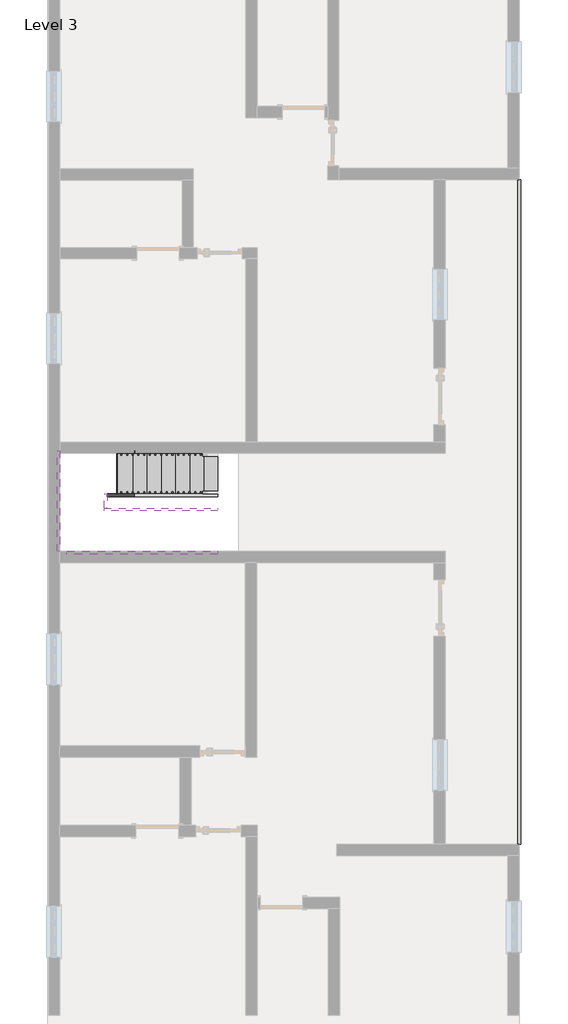
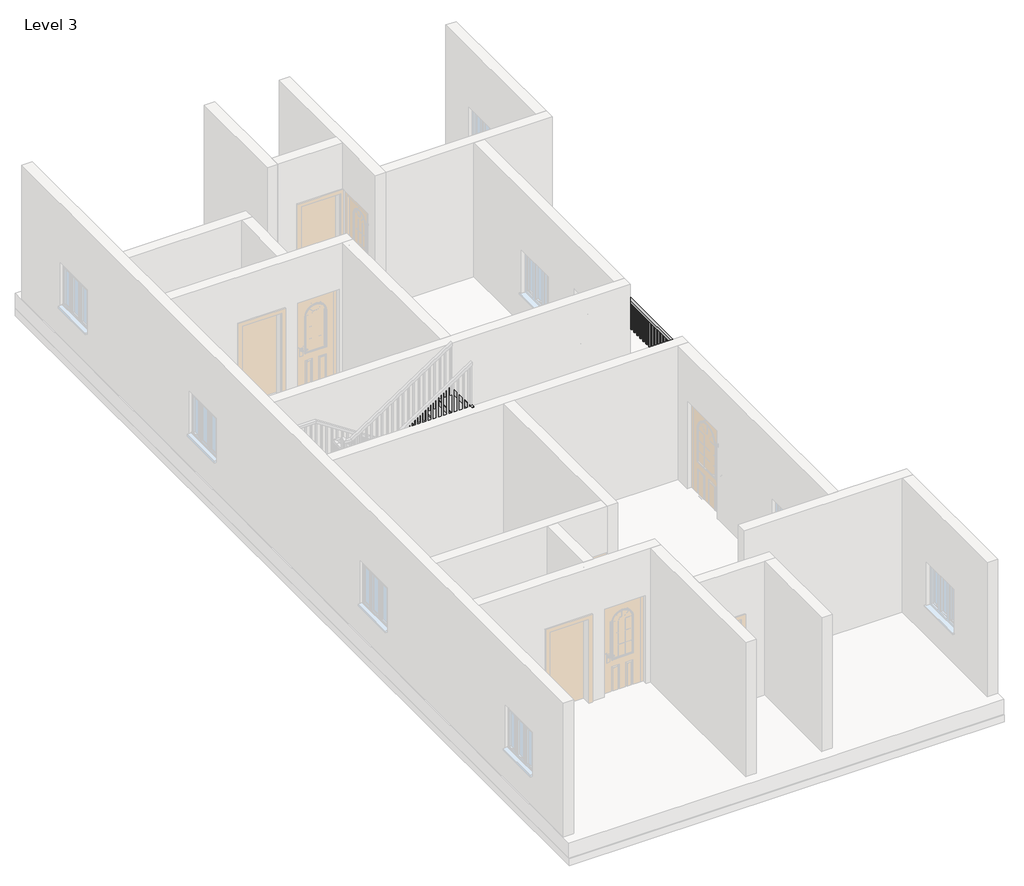
# One storey, part 3 of 3: 6 members, 1 railing, 1 stair flight.
"""IFC4 building model written with IfcOpenShell, lengths in millimetres."""

from ifc_helpers import new_model, si_unit, frame, origin, place, context, project, spatial, polyline, outline, extrude, transform, mapped, element, save
from components import stair_flight_e970c3af

model = new_model("IFC4")

# Units and contexts
model_context = context("Model", 3, world=origin())
ifc_project = project(units=[si_unit("LENGTHUNIT", "METRE", prefix="MILLI")], contexts=[model_context])

# Site, building, storey
site = spatial("IfcSite", under=ifc_project)
building = spatial("IfcBuilding", under=site)
storey = spatial("IfcBuildingStorey", under=building, Name="Level 3", Elevation=6096.0)

# Members
placement = place(None, origin())
element("IfcMember", 1, ObjectType="Stringer - 2\" Width", at=placement, inside=storey, context=model_context, shape_type="SweptSolid", body=[
    extrude(outline(polyline([(6096.0, -2118.1728655), (6313.4747739, -2118.1728655), (7623.2681072, -4099.3728655), (7257.8806735, -4099.3728655), (6096.0, -2341.9063005), (6096.0, -2118.1728655)])), frame((0.0, 417.8797121, 0.0), z_axis=(0.0, 1.0, 0.0), x_axis=(0.0, 0.0, 1.0)), (0.0, 0.0, 1.0), 50.8),
])
element("IfcMember", 2, ObjectType="Stringer - 2\" Width", at=placement, inside=storey, context=model_context, shape_type="SweptSolid", body=[
    extrude(outline(polyline([(-4150.1728655, 468.6797121), (-4099.3728655, 468.6797121), (-4099.3728655, 214.6797121), (-4150.1728655, 214.6797121), (-4150.1728655, 468.6797121)])), frame((0.0, 0.0, 7378.7), z_axis=(0.0, 0.0, 1.0), x_axis=(1.0, 0.0, 0.0)), (0.0, 0.0, 1.0), 304.8),
])
element("IfcMember", 3, ObjectType="Stringer - 2\" Width", at=placement, inside=storey, context=model_context, shape_type="SweptSolid", body=[
    extrude(outline(polyline([(7824.7747739, -4150.1728655), (7459.3873402, -4150.1728655), (8802.765118, -2118.1728655), (9168.1525517, -2118.1728655), (7824.7747739, -4150.1728655)])), frame((0.0, 163.8797121, 0.0), z_axis=(0.0, 1.0, 0.0), x_axis=(0.0, 0.0, 1.0)), (0.0, 0.0, 1.0), 50.8),
])
element("IfcMember", 4, ObjectType="Stringer - 2\" Width", at=placement, inside=storey, context=model_context, shape_type="SweptSolid", body=[
    extrude(outline(polyline([(6096.0, -2118.1728655), (6313.4747739, -2118.1728655), (7683.5, -4190.4799301), (7683.5, -4743.1668047), (6096.0, -2341.9063005), (6096.0, -2118.1728655)])), frame((0.0, 1192.5797121, 0.0), z_axis=(0.0, 1.0, 0.0), x_axis=(0.0, 0.0, 1.0)), (0.0, 0.0, 1.0), 50.8),
])
element("IfcMember", 5, ObjectType="Stringer - 2\" Width", at=placement, inside=storey, context=model_context, shape_type="SweptSolid", body=[
    extrude(outline(polyline([(-4994.7394105, 1243.3797121), (-4943.9394105, 1243.3797121), (-4943.9394105, -560.0202879), (-4994.7394105, -560.0202879), (-4994.7394105, 1243.3797121)])), frame((0.0, 0.0, 7378.7), z_axis=(0.0, 0.0, 1.0), x_axis=(1.0, 0.0, 0.0)), (0.0, 0.0, 1.0), 304.8),
])
element("IfcMember", 6, ObjectType="Stringer - 2\" Width", at=placement, inside=storey, context=model_context, shape_type="SweptSolid", body=[
    extrude(outline(polyline([(7378.7, -4272.2209431), (8802.765118, -2118.1728655), (9168.1525517, -2118.1728655), (7378.7, -4824.9078176), (7378.7, -4272.2209431)])), frame((0.0, -610.8202879, 0.0), z_axis=(0.0, 1.0, 0.0), x_axis=(0.0, 0.0, 1.0)), (0.0, 0.0, 1.0), 50.8),
])

# Railing
element("IfcRailing", 7, ObjectType="Handrail - Rectangular", at=placement, inside=storey, context=model_context, shape_type="SweptSolid", body=[
    extrude(outline(polyline([(3298.3605895, -5805.1202879), (3247.5605895, -5805.1202879), (3247.5605895, 6094.2483916), (3298.3605895, 6094.2483916), (3298.3605895, -5805.1202879)])), frame((0.0, 0.0, 6959.6), z_axis=(0.0, 0.0, 1.0), x_axis=(1.0, 0.0, 0.0)), (0.0, 0.0, 1.0), 50.8),
    extrude(outline(polyline([(3282.4855895, 6072.5547121), (3263.4355895, 6072.5547121), (3263.4355895, 6091.6047121), (3282.4855895, 6091.6047121), (3282.4855895, 6072.5547121)])), frame((0.0, 0.0, 6096.0), z_axis=(0.0, 0.0, 1.0), x_axis=(1.0, 0.0, 0.0)), (0.0, 0.0, 1.0), 863.6),
    extrude(outline(polyline([(3282.4855895, 5970.9547121), (3263.4355895, 5970.9547121), (3263.4355895, 5990.0047121), (3282.4855895, 5990.0047121), (3282.4855895, 5970.9547121)])), frame((0.0, 0.0, 6096.0), z_axis=(0.0, 0.0, 1.0), x_axis=(1.0, 0.0, 0.0)), (0.0, 0.0, 1.0), 863.6),
    extrude(outline(polyline([(3282.4855895, 5869.3547121), (3263.4355895, 5869.3547121), (3263.4355895, 5888.4047121), (3282.4855895, 5888.4047121), (3282.4855895, 5869.3547121)])), frame((0.0, 0.0, 6096.0), z_axis=(0.0, 0.0, 1.0), x_axis=(1.0, 0.0, 0.0)), (0.0, 0.0, 1.0), 863.6),
    extrude(outline(polyline([(3282.4855895, 5767.7547121), (3263.4355895, 5767.7547121), (3263.4355895, 5786.8047121), (3282.4855895, 5786.8047121), (3282.4855895, 5767.7547121)])), frame((0.0, 0.0, 6096.0), z_axis=(0.0, 0.0, 1.0), x_axis=(1.0, 0.0, 0.0)), (0.0, 0.0, 1.0), 863.6),
    extrude(outline(polyline([(3282.4855895, 5666.1547121), (3263.4355895, 5666.1547121), (3263.4355895, 5685.2047121), (3282.4855895, 5685.2047121), (3282.4855895, 5666.1547121)])), frame((0.0, 0.0, 6096.0), z_axis=(0.0, 0.0, 1.0), x_axis=(1.0, 0.0, 0.0)), (0.0, 0.0, 1.0), 863.6),
    extrude(outline(polyline([(3282.4855895, 5564.5547121), (3263.4355895, 5564.5547121), (3263.4355895, 5583.6047121), (3282.4855895, 5583.6047121), (3282.4855895, 5564.5547121)])), frame((0.0, 0.0, 6096.0), z_axis=(0.0, 0.0, 1.0), x_axis=(1.0, 0.0, 0.0)), (0.0, 0.0, 1.0), 863.6),
    extrude(outline(polyline([(3282.4855895, 5462.9547121), (3263.4355895, 5462.9547121), (3263.4355895, 5482.0047121), (3282.4855895, 5482.0047121), (3282.4855895, 5462.9547121)])), frame((0.0, 0.0, 6096.0), z_axis=(0.0, 0.0, 1.0), x_axis=(1.0, 0.0, 0.0)), (0.0, 0.0, 1.0), 863.6),
    extrude(outline(polyline([(3282.4855895, 5361.3547121), (3263.4355895, 5361.3547121), (3263.4355895, 5380.4047121), (3282.4855895, 5380.4047121), (3282.4855895, 5361.3547121)])), frame((0.0, 0.0, 6096.0), z_axis=(0.0, 0.0, 1.0), x_axis=(1.0, 0.0, 0.0)), (0.0, 0.0, 1.0), 863.6),
    extrude(outline(polyline([(3282.4855895, 5259.7547121), (3263.4355895, 5259.7547121), (3263.4355895, 5278.8047121), (3282.4855895, 5278.8047121), (3282.4855895, 5259.7547121)])), frame((0.0, 0.0, 6096.0), z_axis=(0.0, 0.0, 1.0), x_axis=(1.0, 0.0, 0.0)), (0.0, 0.0, 1.0), 863.6),
    extrude(outline(polyline([(3282.4855895, 5158.1547121), (3263.4355895, 5158.1547121), (3263.4355895, 5177.2047121), (3282.4855895, 5177.2047121), (3282.4855895, 5158.1547121)])), frame((0.0, 0.0, 6096.0), z_axis=(0.0, 0.0, 1.0), x_axis=(1.0, 0.0, 0.0)), (0.0, 0.0, 1.0), 863.6),
    extrude(outline(polyline([(3282.4855895, 5056.5547121), (3263.4355895, 5056.5547121), (3263.4355895, 5075.6047121), (3282.4855895, 5075.6047121), (3282.4855895, 5056.5547121)])), frame((0.0, 0.0, 6096.0), z_axis=(0.0, 0.0, 1.0), x_axis=(1.0, 0.0, 0.0)), (0.0, 0.0, 1.0), 863.6),
    extrude(outline(polyline([(3282.4855895, 4954.9547121), (3263.4355895, 4954.9547121), (3263.4355895, 4974.0047121), (3282.4855895, 4974.0047121), (3282.4855895, 4954.9547121)])), frame((0.0, 0.0, 6096.0), z_axis=(0.0, 0.0, 1.0), x_axis=(1.0, 0.0, 0.0)), (0.0, 0.0, 1.0), 863.6),
    extrude(outline(polyline([(3282.4855895, 4853.3547121), (3263.4355895, 4853.3547121), (3263.4355895, 4872.4047121), (3282.4855895, 4872.4047121), (3282.4855895, 4853.3547121)])), frame((0.0, 0.0, 6096.0), z_axis=(0.0, 0.0, 1.0), x_axis=(1.0, 0.0, 0.0)), (0.0, 0.0, 1.0), 863.6),
    extrude(outline(polyline([(3282.4855895, 4751.7547121), (3263.4355895, 4751.7547121), (3263.4355895, 4770.8047121), (3282.4855895, 4770.8047121), (3282.4855895, 4751.7547121)])), frame((0.0, 0.0, 6096.0), z_axis=(0.0, 0.0, 1.0), x_axis=(1.0, 0.0, 0.0)), (0.0, 0.0, 1.0), 863.6),
    extrude(outline(polyline([(3282.4855895, 4650.1547121), (3263.4355895, 4650.1547121), (3263.4355895, 4669.2047121), (3282.4855895, 4669.2047121), (3282.4855895, 4650.1547121)])), frame((0.0, 0.0, 6096.0), z_axis=(0.0, 0.0, 1.0), x_axis=(1.0, 0.0, 0.0)), (0.0, 0.0, 1.0), 863.6),
    extrude(outline(polyline([(3282.4855895, 4548.5547121), (3263.4355895, 4548.5547121), (3263.4355895, 4567.6047121), (3282.4855895, 4567.6047121), (3282.4855895, 4548.5547121)])), frame((0.0, 0.0, 6096.0), z_axis=(0.0, 0.0, 1.0), x_axis=(1.0, 0.0, 0.0)), (0.0, 0.0, 1.0), 863.6),
    extrude(outline(polyline([(3282.4855895, 4446.9547121), (3263.4355895, 4446.9547121), (3263.4355895, 4466.0047121), (3282.4855895, 4466.0047121), (3282.4855895, 4446.9547121)])), frame((0.0, 0.0, 6096.0), z_axis=(0.0, 0.0, 1.0), x_axis=(1.0, 0.0, 0.0)), (0.0, 0.0, 1.0), 863.6),
    extrude(outline(polyline([(3282.4855895, 4345.3547121), (3263.4355895, 4345.3547121), (3263.4355895, 4364.4047121), (3282.4855895, 4364.4047121), (3282.4855895, 4345.3547121)])), frame((0.0, 0.0, 6096.0), z_axis=(0.0, 0.0, 1.0), x_axis=(1.0, 0.0, 0.0)), (0.0, 0.0, 1.0), 863.6),
    extrude(outline(polyline([(3282.4855895, 4243.7547121), (3263.4355895, 4243.7547121), (3263.4355895, 4262.8047121), (3282.4855895, 4262.8047121), (3282.4855895, 4243.7547121)])), frame((0.0, 0.0, 6096.0), z_axis=(0.0, 0.0, 1.0), x_axis=(1.0, 0.0, 0.0)), (0.0, 0.0, 1.0), 863.6),
    extrude(outline(polyline([(3282.4855895, 4142.1547121), (3263.4355895, 4142.1547121), (3263.4355895, 4161.2047121), (3282.4855895, 4161.2047121), (3282.4855895, 4142.1547121)])), frame((0.0, 0.0, 6096.0), z_axis=(0.0, 0.0, 1.0), x_axis=(1.0, 0.0, 0.0)), (0.0, 0.0, 1.0), 863.6),
    extrude(outline(polyline([(3282.4855895, 4040.5547121), (3263.4355895, 4040.5547121), (3263.4355895, 4059.6047121), (3282.4855895, 4059.6047121), (3282.4855895, 4040.5547121)])), frame((0.0, 0.0, 6096.0), z_axis=(0.0, 0.0, 1.0), x_axis=(1.0, 0.0, 0.0)), (0.0, 0.0, 1.0), 863.6),
    extrude(outline(polyline([(3282.4855895, 3938.9547121), (3263.4355895, 3938.9547121), (3263.4355895, 3958.0047121), (3282.4855895, 3958.0047121), (3282.4855895, 3938.9547121)])), frame((0.0, 0.0, 6096.0), z_axis=(0.0, 0.0, 1.0), x_axis=(1.0, 0.0, 0.0)), (0.0, 0.0, 1.0), 863.6),
    extrude(outline(polyline([(3282.4855895, 3837.3547121), (3263.4355895, 3837.3547121), (3263.4355895, 3856.4047121), (3282.4855895, 3856.4047121), (3282.4855895, 3837.3547121)])), frame((0.0, 0.0, 6096.0), z_axis=(0.0, 0.0, 1.0), x_axis=(1.0, 0.0, 0.0)), (0.0, 0.0, 1.0), 863.6),
    extrude(outline(polyline([(3282.4855895, 3735.7547121), (3263.4355895, 3735.7547121), (3263.4355895, 3754.8047121), (3282.4855895, 3754.8047121), (3282.4855895, 3735.7547121)])), frame((0.0, 0.0, 6096.0), z_axis=(0.0, 0.0, 1.0), x_axis=(1.0, 0.0, 0.0)), (0.0, 0.0, 1.0), 863.6),
    extrude(outline(polyline([(3282.4855895, 3634.1547121), (3263.4355895, 3634.1547121), (3263.4355895, 3653.2047121), (3282.4855895, 3653.2047121), (3282.4855895, 3634.1547121)])), frame((0.0, 0.0, 6096.0), z_axis=(0.0, 0.0, 1.0), x_axis=(1.0, 0.0, 0.0)), (0.0, 0.0, 1.0), 863.6),
    extrude(outline(polyline([(3282.4855895, 3532.5547121), (3263.4355895, 3532.5547121), (3263.4355895, 3551.6047121), (3282.4855895, 3551.6047121), (3282.4855895, 3532.5547121)])), frame((0.0, 0.0, 6096.0), z_axis=(0.0, 0.0, 1.0), x_axis=(1.0, 0.0, 0.0)), (0.0, 0.0, 1.0), 863.6),
    extrude(outline(polyline([(3282.4855895, 3430.9547121), (3263.4355895, 3430.9547121), (3263.4355895, 3450.0047121), (3282.4855895, 3450.0047121), (3282.4855895, 3430.9547121)])), frame((0.0, 0.0, 6096.0), z_axis=(0.0, 0.0, 1.0), x_axis=(1.0, 0.0, 0.0)), (0.0, 0.0, 1.0), 863.6),
    extrude(outline(polyline([(3282.4855895, 3329.3547121), (3263.4355895, 3329.3547121), (3263.4355895, 3348.4047121), (3282.4855895, 3348.4047121), (3282.4855895, 3329.3547121)])), frame((0.0, 0.0, 6096.0), z_axis=(0.0, 0.0, 1.0), x_axis=(1.0, 0.0, 0.0)), (0.0, 0.0, 1.0), 863.6),
    extrude(outline(polyline([(3282.4855895, 3227.7547121), (3263.4355895, 3227.7547121), (3263.4355895, 3246.8047121), (3282.4855895, 3246.8047121), (3282.4855895, 3227.7547121)])), frame((0.0, 0.0, 6096.0), z_axis=(0.0, 0.0, 1.0), x_axis=(1.0, 0.0, 0.0)), (0.0, 0.0, 1.0), 863.6),
    extrude(outline(polyline([(3282.4855895, 3126.1547121), (3263.4355895, 3126.1547121), (3263.4355895, 3145.2047121), (3282.4855895, 3145.2047121), (3282.4855895, 3126.1547121)])), frame((0.0, 0.0, 6096.0), z_axis=(0.0, 0.0, 1.0), x_axis=(1.0, 0.0, 0.0)), (0.0, 0.0, 1.0), 863.6),
    extrude(outline(polyline([(3282.4855895, 3024.5547121), (3263.4355895, 3024.5547121), (3263.4355895, 3043.6047121), (3282.4855895, 3043.6047121), (3282.4855895, 3024.5547121)])), frame((0.0, 0.0, 6096.0), z_axis=(0.0, 0.0, 1.0), x_axis=(1.0, 0.0, 0.0)), (0.0, 0.0, 1.0), 863.6),
    extrude(outline(polyline([(3282.4855895, 2922.9547121), (3263.4355895, 2922.9547121), (3263.4355895, 2942.0047121), (3282.4855895, 2942.0047121), (3282.4855895, 2922.9547121)])), frame((0.0, 0.0, 6096.0), z_axis=(0.0, 0.0, 1.0), x_axis=(1.0, 0.0, 0.0)), (0.0, 0.0, 1.0), 863.6),
    extrude(outline(polyline([(3282.4855895, 2821.3547121), (3263.4355895, 2821.3547121), (3263.4355895, 2840.4047121), (3282.4855895, 2840.4047121), (3282.4855895, 2821.3547121)])), frame((0.0, 0.0, 6096.0), z_axis=(0.0, 0.0, 1.0), x_axis=(1.0, 0.0, 0.0)), (0.0, 0.0, 1.0), 863.6),
    extrude(outline(polyline([(3282.4855895, 2719.7547121), (3263.4355895, 2719.7547121), (3263.4355895, 2738.8047121), (3282.4855895, 2738.8047121), (3282.4855895, 2719.7547121)])), frame((0.0, 0.0, 6096.0), z_axis=(0.0, 0.0, 1.0), x_axis=(1.0, 0.0, 0.0)), (0.0, 0.0, 1.0), 863.6),
    extrude(outline(polyline([(3282.4855895, 2618.1547121), (3263.4355895, 2618.1547121), (3263.4355895, 2637.2047121), (3282.4855895, 2637.2047121), (3282.4855895, 2618.1547121)])), frame((0.0, 0.0, 6096.0), z_axis=(0.0, 0.0, 1.0), x_axis=(1.0, 0.0, 0.0)), (0.0, 0.0, 1.0), 863.6),
    extrude(outline(polyline([(3282.4855895, 2516.5547121), (3263.4355895, 2516.5547121), (3263.4355895, 2535.6047121), (3282.4855895, 2535.6047121), (3282.4855895, 2516.5547121)])), frame((0.0, 0.0, 6096.0), z_axis=(0.0, 0.0, 1.0), x_axis=(1.0, 0.0, 0.0)), (0.0, 0.0, 1.0), 863.6),
    extrude(outline(polyline([(3282.4855895, 2414.9547121), (3263.4355895, 2414.9547121), (3263.4355895, 2434.0047121), (3282.4855895, 2434.0047121), (3282.4855895, 2414.9547121)])), frame((0.0, 0.0, 6096.0), z_axis=(0.0, 0.0, 1.0), x_axis=(1.0, 0.0, 0.0)), (0.0, 0.0, 1.0), 863.6),
    extrude(outline(polyline([(3282.4855895, 2313.3547121), (3263.4355895, 2313.3547121), (3263.4355895, 2332.4047121), (3282.4855895, 2332.4047121), (3282.4855895, 2313.3547121)])), frame((0.0, 0.0, 6096.0), z_axis=(0.0, 0.0, 1.0), x_axis=(1.0, 0.0, 0.0)), (0.0, 0.0, 1.0), 863.6),
    extrude(outline(polyline([(3282.4855895, 2211.7547121), (3263.4355895, 2211.7547121), (3263.4355895, 2230.8047121), (3282.4855895, 2230.8047121), (3282.4855895, 2211.7547121)])), frame((0.0, 0.0, 6096.0), z_axis=(0.0, 0.0, 1.0), x_axis=(1.0, 0.0, 0.0)), (0.0, 0.0, 1.0), 863.6),
    extrude(outline(polyline([(3282.4855895, 2110.1547121), (3263.4355895, 2110.1547121), (3263.4355895, 2129.2047121), (3282.4855895, 2129.2047121), (3282.4855895, 2110.1547121)])), frame((0.0, 0.0, 6096.0), z_axis=(0.0, 0.0, 1.0), x_axis=(1.0, 0.0, 0.0)), (0.0, 0.0, 1.0), 863.6),
    extrude(outline(polyline([(3282.4855895, 2008.5547121), (3263.4355895, 2008.5547121), (3263.4355895, 2027.6047121), (3282.4855895, 2027.6047121), (3282.4855895, 2008.5547121)])), frame((0.0, 0.0, 6096.0), z_axis=(0.0, 0.0, 1.0), x_axis=(1.0, 0.0, 0.0)), (0.0, 0.0, 1.0), 863.6),
    extrude(outline(polyline([(3282.4855895, 1906.9547121), (3263.4355895, 1906.9547121), (3263.4355895, 1926.0047121), (3282.4855895, 1926.0047121), (3282.4855895, 1906.9547121)])), frame((0.0, 0.0, 6096.0), z_axis=(0.0, 0.0, 1.0), x_axis=(1.0, 0.0, 0.0)), (0.0, 0.0, 1.0), 863.6),
    extrude(outline(polyline([(3282.4855895, 1805.3547121), (3263.4355895, 1805.3547121), (3263.4355895, 1824.4047121), (3282.4855895, 1824.4047121), (3282.4855895, 1805.3547121)])), frame((0.0, 0.0, 6096.0), z_axis=(0.0, 0.0, 1.0), x_axis=(1.0, 0.0, 0.0)), (0.0, 0.0, 1.0), 863.6),
    extrude(outline(polyline([(3282.4855895, 1703.7547121), (3263.4355895, 1703.7547121), (3263.4355895, 1722.8047121), (3282.4855895, 1722.8047121), (3282.4855895, 1703.7547121)])), frame((0.0, 0.0, 6096.0), z_axis=(0.0, 0.0, 1.0), x_axis=(1.0, 0.0, 0.0)), (0.0, 0.0, 1.0), 863.6),
    extrude(outline(polyline([(3282.4855895, 1602.1547121), (3263.4355895, 1602.1547121), (3263.4355895, 1621.2047121), (3282.4855895, 1621.2047121), (3282.4855895, 1602.1547121)])), frame((0.0, 0.0, 6096.0), z_axis=(0.0, 0.0, 1.0), x_axis=(1.0, 0.0, 0.0)), (0.0, 0.0, 1.0), 863.6),
    extrude(outline(polyline([(3282.4855895, 1500.5547121), (3263.4355895, 1500.5547121), (3263.4355895, 1519.6047121), (3282.4855895, 1519.6047121), (3282.4855895, 1500.5547121)])), frame((0.0, 0.0, 6096.0), z_axis=(0.0, 0.0, 1.0), x_axis=(1.0, 0.0, 0.0)), (0.0, 0.0, 1.0), 863.6),
    extrude(outline(polyline([(3282.4855895, 1398.9547121), (3263.4355895, 1398.9547121), (3263.4355895, 1418.0047121), (3282.4855895, 1418.0047121), (3282.4855895, 1398.9547121)])), frame((0.0, 0.0, 6096.0), z_axis=(0.0, 0.0, 1.0), x_axis=(1.0, 0.0, 0.0)), (0.0, 0.0, 1.0), 863.6),
    extrude(outline(polyline([(3282.4855895, 1297.3547121), (3263.4355895, 1297.3547121), (3263.4355895, 1316.4047121), (3282.4855895, 1316.4047121), (3282.4855895, 1297.3547121)])), frame((0.0, 0.0, 6096.0), z_axis=(0.0, 0.0, 1.0), x_axis=(1.0, 0.0, 0.0)), (0.0, 0.0, 1.0), 863.6),
    extrude(outline(polyline([(3282.4855895, 1195.7547121), (3263.4355895, 1195.7547121), (3263.4355895, 1214.8047121), (3282.4855895, 1214.8047121), (3282.4855895, 1195.7547121)])), frame((0.0, 0.0, 6096.0), z_axis=(0.0, 0.0, 1.0), x_axis=(1.0, 0.0, 0.0)), (0.0, 0.0, 1.0), 863.6),
    extrude(outline(polyline([(3282.4855895, 1094.1547121), (3263.4355895, 1094.1547121), (3263.4355895, 1113.2047121), (3282.4855895, 1113.2047121), (3282.4855895, 1094.1547121)])), frame((0.0, 0.0, 6096.0), z_axis=(0.0, 0.0, 1.0), x_axis=(1.0, 0.0, 0.0)), (0.0, 0.0, 1.0), 863.6),
    extrude(outline(polyline([(3282.4855895, 992.5547121), (3263.4355895, 992.5547121), (3263.4355895, 1011.6047121), (3282.4855895, 1011.6047121), (3282.4855895, 992.5547121)])), frame((0.0, 0.0, 6096.0), z_axis=(0.0, 0.0, 1.0), x_axis=(1.0, 0.0, 0.0)), (0.0, 0.0, 1.0), 863.6),
    extrude(outline(polyline([(3282.4855895, 890.9547121), (3263.4355895, 890.9547121), (3263.4355895, 910.0047121), (3282.4855895, 910.0047121), (3282.4855895, 890.9547121)])), frame((0.0, 0.0, 6096.0), z_axis=(0.0, 0.0, 1.0), x_axis=(1.0, 0.0, 0.0)), (0.0, 0.0, 1.0), 863.6),
    extrude(outline(polyline([(3282.4855895, 789.3547121), (3263.4355895, 789.3547121), (3263.4355895, 808.4047121), (3282.4855895, 808.4047121), (3282.4855895, 789.3547121)])), frame((0.0, 0.0, 6096.0), z_axis=(0.0, 0.0, 1.0), x_axis=(1.0, 0.0, 0.0)), (0.0, 0.0, 1.0), 863.6),
    extrude(outline(polyline([(3282.4855895, 687.7547121), (3263.4355895, 687.7547121), (3263.4355895, 706.8047121), (3282.4855895, 706.8047121), (3282.4855895, 687.7547121)])), frame((0.0, 0.0, 6096.0), z_axis=(0.0, 0.0, 1.0), x_axis=(1.0, 0.0, 0.0)), (0.0, 0.0, 1.0), 863.6),
    extrude(outline(polyline([(3282.4855895, 586.1547121), (3263.4355895, 586.1547121), (3263.4355895, 605.2047121), (3282.4855895, 605.2047121), (3282.4855895, 586.1547121)])), frame((0.0, 0.0, 6096.0), z_axis=(0.0, 0.0, 1.0), x_axis=(1.0, 0.0, 0.0)), (0.0, 0.0, 1.0), 863.6),
    extrude(outline(polyline([(3282.4855895, 484.5547121), (3263.4355895, 484.5547121), (3263.4355895, 503.6047121), (3282.4855895, 503.6047121), (3282.4855895, 484.5547121)])), frame((0.0, 0.0, 6096.0), z_axis=(0.0, 0.0, 1.0), x_axis=(1.0, 0.0, 0.0)), (0.0, 0.0, 1.0), 863.6),
    extrude(outline(polyline([(3282.4855895, 382.9547121), (3263.4355895, 382.9547121), (3263.4355895, 402.0047121), (3282.4855895, 402.0047121), (3282.4855895, 382.9547121)])), frame((0.0, 0.0, 6096.0), z_axis=(0.0, 0.0, 1.0), x_axis=(1.0, 0.0, 0.0)), (0.0, 0.0, 1.0), 863.6),
    extrude(outline(polyline([(3282.4855895, 281.3547121), (3263.4355895, 281.3547121), (3263.4355895, 300.4047121), (3282.4855895, 300.4047121), (3282.4855895, 281.3547121)])), frame((0.0, 0.0, 6096.0), z_axis=(0.0, 0.0, 1.0), x_axis=(1.0, 0.0, 0.0)), (0.0, 0.0, 1.0), 863.6),
    extrude(outline(polyline([(3282.4855895, 179.7547121), (3263.4355895, 179.7547121), (3263.4355895, 198.8047121), (3282.4855895, 198.8047121), (3282.4855895, 179.7547121)])), frame((0.0, 0.0, 6096.0), z_axis=(0.0, 0.0, 1.0), x_axis=(1.0, 0.0, 0.0)), (0.0, 0.0, 1.0), 863.6),
    extrude(outline(polyline([(3282.4855895, 78.1547121), (3263.4355895, 78.1547121), (3263.4355895, 97.2047121), (3282.4855895, 97.2047121), (3282.4855895, 78.1547121)])), frame((0.0, 0.0, 6096.0), z_axis=(0.0, 0.0, 1.0), x_axis=(1.0, 0.0, 0.0)), (0.0, 0.0, 1.0), 863.6),
    extrude(outline(polyline([(3282.4855895, -23.4452879), (3263.4355895, -23.4452879), (3263.4355895, -4.3952879), (3282.4855895, -4.3952879), (3282.4855895, -23.4452879)])), frame((0.0, 0.0, 6096.0), z_axis=(0.0, 0.0, 1.0), x_axis=(1.0, 0.0, 0.0)), (0.0, 0.0, 1.0), 863.6),
    extrude(outline(polyline([(3282.4855895, -125.0452879), (3263.4355895, -125.0452879), (3263.4355895, -105.9952879), (3282.4855895, -105.9952879), (3282.4855895, -125.0452879)])), frame((0.0, 0.0, 6096.0), z_axis=(0.0, 0.0, 1.0), x_axis=(1.0, 0.0, 0.0)), (0.0, 0.0, 1.0), 863.6),
    extrude(outline(polyline([(3282.4855895, -226.6452879), (3263.4355895, -226.6452879), (3263.4355895, -207.5952879), (3282.4855895, -207.5952879), (3282.4855895, -226.6452879)])), frame((0.0, 0.0, 6096.0), z_axis=(0.0, 0.0, 1.0), x_axis=(1.0, 0.0, 0.0)), (0.0, 0.0, 1.0), 863.6),
    extrude(outline(polyline([(3282.4855895, -328.2452879), (3263.4355895, -328.2452879), (3263.4355895, -309.1952879), (3282.4855895, -309.1952879), (3282.4855895, -328.2452879)])), frame((0.0, 0.0, 6096.0), z_axis=(0.0, 0.0, 1.0), x_axis=(1.0, 0.0, 0.0)), (0.0, 0.0, 1.0), 863.6),
    extrude(outline(polyline([(3282.4855895, -429.8452879), (3263.4355895, -429.8452879), (3263.4355895, -410.7952879), (3282.4855895, -410.7952879), (3282.4855895, -429.8452879)])), frame((0.0, 0.0, 6096.0), z_axis=(0.0, 0.0, 1.0), x_axis=(1.0, 0.0, 0.0)), (0.0, 0.0, 1.0), 863.6),
    extrude(outline(polyline([(3282.4855895, -531.4452879), (3263.4355895, -531.4452879), (3263.4355895, -512.3952879), (3282.4855895, -512.3952879), (3282.4855895, -531.4452879)])), frame((0.0, 0.0, 6096.0), z_axis=(0.0, 0.0, 1.0), x_axis=(1.0, 0.0, 0.0)), (0.0, 0.0, 1.0), 863.6),
    extrude(outline(polyline([(3282.4855895, -633.0452879), (3263.4355895, -633.0452879), (3263.4355895, -613.9952879), (3282.4855895, -613.9952879), (3282.4855895, -633.0452879)])), frame((0.0, 0.0, 6096.0), z_axis=(0.0, 0.0, 1.0), x_axis=(1.0, 0.0, 0.0)), (0.0, 0.0, 1.0), 863.6),
    extrude(outline(polyline([(3282.4855895, -734.6452879), (3263.4355895, -734.6452879), (3263.4355895, -715.5952879), (3282.4855895, -715.5952879), (3282.4855895, -734.6452879)])), frame((0.0, 0.0, 6096.0), z_axis=(0.0, 0.0, 1.0), x_axis=(1.0, 0.0, 0.0)), (0.0, 0.0, 1.0), 863.6),
    extrude(outline(polyline([(3282.4855895, -836.2452879), (3263.4355895, -836.2452879), (3263.4355895, -817.1952879), (3282.4855895, -817.1952879), (3282.4855895, -836.2452879)])), frame((0.0, 0.0, 6096.0), z_axis=(0.0, 0.0, 1.0), x_axis=(1.0, 0.0, 0.0)), (0.0, 0.0, 1.0), 863.6),
    extrude(outline(polyline([(3282.4855895, -937.8452879), (3263.4355895, -937.8452879), (3263.4355895, -918.7952879), (3282.4855895, -918.7952879), (3282.4855895, -937.8452879)])), frame((0.0, 0.0, 6096.0), z_axis=(0.0, 0.0, 1.0), x_axis=(1.0, 0.0, 0.0)), (0.0, 0.0, 1.0), 863.6),
    extrude(outline(polyline([(3282.4855895, -1039.4452879), (3263.4355895, -1039.4452879), (3263.4355895, -1020.3952879), (3282.4855895, -1020.3952879), (3282.4855895, -1039.4452879)])), frame((0.0, 0.0, 6096.0), z_axis=(0.0, 0.0, 1.0), x_axis=(1.0, 0.0, 0.0)), (0.0, 0.0, 1.0), 863.6),
    extrude(outline(polyline([(3282.4855895, -1141.0452879), (3263.4355895, -1141.0452879), (3263.4355895, -1121.9952879), (3282.4855895, -1121.9952879), (3282.4855895, -1141.0452879)])), frame((0.0, 0.0, 6096.0), z_axis=(0.0, 0.0, 1.0), x_axis=(1.0, 0.0, 0.0)), (0.0, 0.0, 1.0), 863.6),
    extrude(outline(polyline([(3282.4855895, -1242.6452879), (3263.4355895, -1242.6452879), (3263.4355895, -1223.5952879), (3282.4855895, -1223.5952879), (3282.4855895, -1242.6452879)])), frame((0.0, 0.0, 6096.0), z_axis=(0.0, 0.0, 1.0), x_axis=(1.0, 0.0, 0.0)), (0.0, 0.0, 1.0), 863.6),
    extrude(outline(polyline([(3282.4855895, -1344.2452879), (3263.4355895, -1344.2452879), (3263.4355895, -1325.1952879), (3282.4855895, -1325.1952879), (3282.4855895, -1344.2452879)])), frame((0.0, 0.0, 6096.0), z_axis=(0.0, 0.0, 1.0), x_axis=(1.0, 0.0, 0.0)), (0.0, 0.0, 1.0), 863.6),
    extrude(outline(polyline([(3282.4855895, -1445.8452879), (3263.4355895, -1445.8452879), (3263.4355895, -1426.7952879), (3282.4855895, -1426.7952879), (3282.4855895, -1445.8452879)])), frame((0.0, 0.0, 6096.0), z_axis=(0.0, 0.0, 1.0), x_axis=(1.0, 0.0, 0.0)), (0.0, 0.0, 1.0), 863.6),
    extrude(outline(polyline([(3282.4855895, -1547.4452879), (3263.4355895, -1547.4452879), (3263.4355895, -1528.3952879), (3282.4855895, -1528.3952879), (3282.4855895, -1547.4452879)])), frame((0.0, 0.0, 6096.0), z_axis=(0.0, 0.0, 1.0), x_axis=(1.0, 0.0, 0.0)), (0.0, 0.0, 1.0), 863.6),
    extrude(outline(polyline([(3282.4855895, -1649.0452879), (3263.4355895, -1649.0452879), (3263.4355895, -1629.9952879), (3282.4855895, -1629.9952879), (3282.4855895, -1649.0452879)])), frame((0.0, 0.0, 6096.0), z_axis=(0.0, 0.0, 1.0), x_axis=(1.0, 0.0, 0.0)), (0.0, 0.0, 1.0), 863.6),
    extrude(outline(polyline([(3282.4855895, -1750.6452879), (3263.4355895, -1750.6452879), (3263.4355895, -1731.5952879), (3282.4855895, -1731.5952879), (3282.4855895, -1750.6452879)])), frame((0.0, 0.0, 6096.0), z_axis=(0.0, 0.0, 1.0), x_axis=(1.0, 0.0, 0.0)), (0.0, 0.0, 1.0), 863.6),
    extrude(outline(polyline([(3282.4855895, -1852.2452879), (3263.4355895, -1852.2452879), (3263.4355895, -1833.1952879), (3282.4855895, -1833.1952879), (3282.4855895, -1852.2452879)])), frame((0.0, 0.0, 6096.0), z_axis=(0.0, 0.0, 1.0), x_axis=(1.0, 0.0, 0.0)), (0.0, 0.0, 1.0), 863.6),
    extrude(outline(polyline([(3282.4855895, -1953.8452879), (3263.4355895, -1953.8452879), (3263.4355895, -1934.7952879), (3282.4855895, -1934.7952879), (3282.4855895, -1953.8452879)])), frame((0.0, 0.0, 6096.0), z_axis=(0.0, 0.0, 1.0), x_axis=(1.0, 0.0, 0.0)), (0.0, 0.0, 1.0), 863.6),
    extrude(outline(polyline([(3282.4855895, -2055.4452879), (3263.4355895, -2055.4452879), (3263.4355895, -2036.3952879), (3282.4855895, -2036.3952879), (3282.4855895, -2055.4452879)])), frame((0.0, 0.0, 6096.0), z_axis=(0.0, 0.0, 1.0), x_axis=(1.0, 0.0, 0.0)), (0.0, 0.0, 1.0), 863.6),
    extrude(outline(polyline([(3282.4855895, -2157.0452879), (3263.4355895, -2157.0452879), (3263.4355895, -2137.9952879), (3282.4855895, -2137.9952879), (3282.4855895, -2157.0452879)])), frame((0.0, 0.0, 6096.0), z_axis=(0.0, 0.0, 1.0), x_axis=(1.0, 0.0, 0.0)), (0.0, 0.0, 1.0), 863.6),
    extrude(outline(polyline([(3282.4855895, -2258.6452879), (3263.4355895, -2258.6452879), (3263.4355895, -2239.5952879), (3282.4855895, -2239.5952879), (3282.4855895, -2258.6452879)])), frame((0.0, 0.0, 6096.0), z_axis=(0.0, 0.0, 1.0), x_axis=(1.0, 0.0, 0.0)), (0.0, 0.0, 1.0), 863.6),
    extrude(outline(polyline([(3282.4855895, -2360.2452879), (3263.4355895, -2360.2452879), (3263.4355895, -2341.1952879), (3282.4855895, -2341.1952879), (3282.4855895, -2360.2452879)])), frame((0.0, 0.0, 6096.0), z_axis=(0.0, 0.0, 1.0), x_axis=(1.0, 0.0, 0.0)), (0.0, 0.0, 1.0), 863.6),
    extrude(outline(polyline([(3282.4855895, -2461.8452879), (3263.4355895, -2461.8452879), (3263.4355895, -2442.7952879), (3282.4855895, -2442.7952879), (3282.4855895, -2461.8452879)])), frame((0.0, 0.0, 6096.0), z_axis=(0.0, 0.0, 1.0), x_axis=(1.0, 0.0, 0.0)), (0.0, 0.0, 1.0), 863.6),
    extrude(outline(polyline([(3282.4855895, -2563.4452879), (3263.4355895, -2563.4452879), (3263.4355895, -2544.3952879), (3282.4855895, -2544.3952879), (3282.4855895, -2563.4452879)])), frame((0.0, 0.0, 6096.0), z_axis=(0.0, 0.0, 1.0), x_axis=(1.0, 0.0, 0.0)), (0.0, 0.0, 1.0), 863.6),
    extrude(outline(polyline([(3282.4855895, -2665.0452879), (3263.4355895, -2665.0452879), (3263.4355895, -2645.9952879), (3282.4855895, -2645.9952879), (3282.4855895, -2665.0452879)])), frame((0.0, 0.0, 6096.0), z_axis=(0.0, 0.0, 1.0), x_axis=(1.0, 0.0, 0.0)), (0.0, 0.0, 1.0), 863.6),
    extrude(outline(polyline([(3282.4855895, -2766.6452879), (3263.4355895, -2766.6452879), (3263.4355895, -2747.5952879), (3282.4855895, -2747.5952879), (3282.4855895, -2766.6452879)])), frame((0.0, 0.0, 6096.0), z_axis=(0.0, 0.0, 1.0), x_axis=(1.0, 0.0, 0.0)), (0.0, 0.0, 1.0), 863.6),
    extrude(outline(polyline([(3282.4855895, -2868.2452879), (3263.4355895, -2868.2452879), (3263.4355895, -2849.1952879), (3282.4855895, -2849.1952879), (3282.4855895, -2868.2452879)])), frame((0.0, 0.0, 6096.0), z_axis=(0.0, 0.0, 1.0), x_axis=(1.0, 0.0, 0.0)), (0.0, 0.0, 1.0), 863.6),
    extrude(outline(polyline([(3282.4855895, -2969.8452879), (3263.4355895, -2969.8452879), (3263.4355895, -2950.7952879), (3282.4855895, -2950.7952879), (3282.4855895, -2969.8452879)])), frame((0.0, 0.0, 6096.0), z_axis=(0.0, 0.0, 1.0), x_axis=(1.0, 0.0, 0.0)), (0.0, 0.0, 1.0), 863.6),
    extrude(outline(polyline([(3282.4855895, -3071.4452879), (3263.4355895, -3071.4452879), (3263.4355895, -3052.3952879), (3282.4855895, -3052.3952879), (3282.4855895, -3071.4452879)])), frame((0.0, 0.0, 6096.0), z_axis=(0.0, 0.0, 1.0), x_axis=(1.0, 0.0, 0.0)), (0.0, 0.0, 1.0), 863.6),
    extrude(outline(polyline([(3282.4855895, -3173.0452879), (3263.4355895, -3173.0452879), (3263.4355895, -3153.9952879), (3282.4855895, -3153.9952879), (3282.4855895, -3173.0452879)])), frame((0.0, 0.0, 6096.0), z_axis=(0.0, 0.0, 1.0), x_axis=(1.0, 0.0, 0.0)), (0.0, 0.0, 1.0), 863.6),
    extrude(outline(polyline([(3282.4855895, -3274.6452879), (3263.4355895, -3274.6452879), (3263.4355895, -3255.5952879), (3282.4855895, -3255.5952879), (3282.4855895, -3274.6452879)])), frame((0.0, 0.0, 6096.0), z_axis=(0.0, 0.0, 1.0), x_axis=(1.0, 0.0, 0.0)), (0.0, 0.0, 1.0), 863.6),
    extrude(outline(polyline([(3282.4855895, -3376.2452879), (3263.4355895, -3376.2452879), (3263.4355895, -3357.1952879), (3282.4855895, -3357.1952879), (3282.4855895, -3376.2452879)])), frame((0.0, 0.0, 6096.0), z_axis=(0.0, 0.0, 1.0), x_axis=(1.0, 0.0, 0.0)), (0.0, 0.0, 1.0), 863.6),
    extrude(outline(polyline([(3282.4855895, -3477.8452879), (3263.4355895, -3477.8452879), (3263.4355895, -3458.7952879), (3282.4855895, -3458.7952879), (3282.4855895, -3477.8452879)])), frame((0.0, 0.0, 6096.0), z_axis=(0.0, 0.0, 1.0), x_axis=(1.0, 0.0, 0.0)), (0.0, 0.0, 1.0), 863.6),
    extrude(outline(polyline([(3282.4855895, -3579.4452879), (3263.4355895, -3579.4452879), (3263.4355895, -3560.3952879), (3282.4855895, -3560.3952879), (3282.4855895, -3579.4452879)])), frame((0.0, 0.0, 6096.0), z_axis=(0.0, 0.0, 1.0), x_axis=(1.0, 0.0, 0.0)), (0.0, 0.0, 1.0), 863.6),
    extrude(outline(polyline([(3282.4855895, -3681.0452879), (3263.4355895, -3681.0452879), (3263.4355895, -3661.9952879), (3282.4855895, -3661.9952879), (3282.4855895, -3681.0452879)])), frame((0.0, 0.0, 6096.0), z_axis=(0.0, 0.0, 1.0), x_axis=(1.0, 0.0, 0.0)), (0.0, 0.0, 1.0), 863.6),
    extrude(outline(polyline([(3282.4855895, -3782.6452879), (3263.4355895, -3782.6452879), (3263.4355895, -3763.5952879), (3282.4855895, -3763.5952879), (3282.4855895, -3782.6452879)])), frame((0.0, 0.0, 6096.0), z_axis=(0.0, 0.0, 1.0), x_axis=(1.0, 0.0, 0.0)), (0.0, 0.0, 1.0), 863.6),
    extrude(outline(polyline([(3282.4855895, -3884.2452879), (3263.4355895, -3884.2452879), (3263.4355895, -3865.1952879), (3282.4855895, -3865.1952879), (3282.4855895, -3884.2452879)])), frame((0.0, 0.0, 6096.0), z_axis=(0.0, 0.0, 1.0), x_axis=(1.0, 0.0, 0.0)), (0.0, 0.0, 1.0), 863.6),
    extrude(outline(polyline([(3282.4855895, -3985.8452879), (3263.4355895, -3985.8452879), (3263.4355895, -3966.7952879), (3282.4855895, -3966.7952879), (3282.4855895, -3985.8452879)])), frame((0.0, 0.0, 6096.0), z_axis=(0.0, 0.0, 1.0), x_axis=(1.0, 0.0, 0.0)), (0.0, 0.0, 1.0), 863.6),
    extrude(outline(polyline([(3282.4855895, -4087.4452879), (3263.4355895, -4087.4452879), (3263.4355895, -4068.3952879), (3282.4855895, -4068.3952879), (3282.4855895, -4087.4452879)])), frame((0.0, 0.0, 6096.0), z_axis=(0.0, 0.0, 1.0), x_axis=(1.0, 0.0, 0.0)), (0.0, 0.0, 1.0), 863.6),
    extrude(outline(polyline([(3282.4855895, -4189.0452879), (3263.4355895, -4189.0452879), (3263.4355895, -4169.9952879), (3282.4855895, -4169.9952879), (3282.4855895, -4189.0452879)])), frame((0.0, 0.0, 6096.0), z_axis=(0.0, 0.0, 1.0), x_axis=(1.0, 0.0, 0.0)), (0.0, 0.0, 1.0), 863.6),
    extrude(outline(polyline([(3282.4855895, -4290.6452879), (3263.4355895, -4290.6452879), (3263.4355895, -4271.5952879), (3282.4855895, -4271.5952879), (3282.4855895, -4290.6452879)])), frame((0.0, 0.0, 6096.0), z_axis=(0.0, 0.0, 1.0), x_axis=(1.0, 0.0, 0.0)), (0.0, 0.0, 1.0), 863.6),
    extrude(outline(polyline([(3282.4855895, -4392.2452879), (3263.4355895, -4392.2452879), (3263.4355895, -4373.1952879), (3282.4855895, -4373.1952879), (3282.4855895, -4392.2452879)])), frame((0.0, 0.0, 6096.0), z_axis=(0.0, 0.0, 1.0), x_axis=(1.0, 0.0, 0.0)), (0.0, 0.0, 1.0), 863.6),
    extrude(outline(polyline([(3282.4855895, -4493.8452879), (3263.4355895, -4493.8452879), (3263.4355895, -4474.7952879), (3282.4855895, -4474.7952879), (3282.4855895, -4493.8452879)])), frame((0.0, 0.0, 6096.0), z_axis=(0.0, 0.0, 1.0), x_axis=(1.0, 0.0, 0.0)), (0.0, 0.0, 1.0), 863.6),
    extrude(outline(polyline([(3282.4855895, -4595.4452879), (3263.4355895, -4595.4452879), (3263.4355895, -4576.3952879), (3282.4855895, -4576.3952879), (3282.4855895, -4595.4452879)])), frame((0.0, 0.0, 6096.0), z_axis=(0.0, 0.0, 1.0), x_axis=(1.0, 0.0, 0.0)), (0.0, 0.0, 1.0), 863.6),
    extrude(outline(polyline([(3282.4855895, -4697.0452879), (3263.4355895, -4697.0452879), (3263.4355895, -4677.9952879), (3282.4855895, -4677.9952879), (3282.4855895, -4697.0452879)])), frame((0.0, 0.0, 6096.0), z_axis=(0.0, 0.0, 1.0), x_axis=(1.0, 0.0, 0.0)), (0.0, 0.0, 1.0), 863.6),
    extrude(outline(polyline([(3282.4855895, -4798.6452879), (3263.4355895, -4798.6452879), (3263.4355895, -4779.5952879), (3282.4855895, -4779.5952879), (3282.4855895, -4798.6452879)])), frame((0.0, 0.0, 6096.0), z_axis=(0.0, 0.0, 1.0), x_axis=(1.0, 0.0, 0.0)), (0.0, 0.0, 1.0), 863.6),
    extrude(outline(polyline([(3282.4855895, -4900.2452879), (3263.4355895, -4900.2452879), (3263.4355895, -4881.1952879), (3282.4855895, -4881.1952879), (3282.4855895, -4900.2452879)])), frame((0.0, 0.0, 6096.0), z_axis=(0.0, 0.0, 1.0), x_axis=(1.0, 0.0, 0.0)), (0.0, 0.0, 1.0), 863.6),
    extrude(outline(polyline([(3282.4855895, -5001.8452879), (3263.4355895, -5001.8452879), (3263.4355895, -4982.7952879), (3282.4855895, -4982.7952879), (3282.4855895, -5001.8452879)])), frame((0.0, 0.0, 6096.0), z_axis=(0.0, 0.0, 1.0), x_axis=(1.0, 0.0, 0.0)), (0.0, 0.0, 1.0), 863.6),
    extrude(outline(polyline([(3282.4855895, -5103.4452879), (3263.4355895, -5103.4452879), (3263.4355895, -5084.3952879), (3282.4855895, -5084.3952879), (3282.4855895, -5103.4452879)])), frame((0.0, 0.0, 6096.0), z_axis=(0.0, 0.0, 1.0), x_axis=(1.0, 0.0, 0.0)), (0.0, 0.0, 1.0), 863.6),
    extrude(outline(polyline([(3282.4855895, -5205.0452879), (3263.4355895, -5205.0452879), (3263.4355895, -5185.9952879), (3282.4855895, -5185.9952879), (3282.4855895, -5205.0452879)])), frame((0.0, 0.0, 6096.0), z_axis=(0.0, 0.0, 1.0), x_axis=(1.0, 0.0, 0.0)), (0.0, 0.0, 1.0), 863.6),
    extrude(outline(polyline([(3282.4855895, -5306.6452879), (3263.4355895, -5306.6452879), (3263.4355895, -5287.5952879), (3282.4855895, -5287.5952879), (3282.4855895, -5306.6452879)])), frame((0.0, 0.0, 6096.0), z_axis=(0.0, 0.0, 1.0), x_axis=(1.0, 0.0, 0.0)), (0.0, 0.0, 1.0), 863.6),
    extrude(outline(polyline([(3282.4855895, -5408.2452879), (3263.4355895, -5408.2452879), (3263.4355895, -5389.1952879), (3282.4855895, -5389.1952879), (3282.4855895, -5408.2452879)])), frame((0.0, 0.0, 6096.0), z_axis=(0.0, 0.0, 1.0), x_axis=(1.0, 0.0, 0.0)), (0.0, 0.0, 1.0), 863.6),
    extrude(outline(polyline([(3282.4855895, -5509.8452879), (3263.4355895, -5509.8452879), (3263.4355895, -5490.7952879), (3282.4855895, -5490.7952879), (3282.4855895, -5509.8452879)])), frame((0.0, 0.0, 6096.0), z_axis=(0.0, 0.0, 1.0), x_axis=(1.0, 0.0, 0.0)), (0.0, 0.0, 1.0), 863.6),
    extrude(outline(polyline([(3282.4855895, -5611.4452879), (3263.4355895, -5611.4452879), (3263.4355895, -5592.3952879), (3282.4855895, -5592.3952879), (3282.4855895, -5611.4452879)])), frame((0.0, 0.0, 6096.0), z_axis=(0.0, 0.0, 1.0), x_axis=(1.0, 0.0, 0.0)), (0.0, 0.0, 1.0), 863.6),
    extrude(outline(polyline([(3282.4855895, -5713.0452879), (3263.4355895, -5713.0452879), (3263.4355895, -5693.9952879), (3282.4855895, -5693.9952879), (3282.4855895, -5713.0452879)])), frame((0.0, 0.0, 6096.0), z_axis=(0.0, 0.0, 1.0), x_axis=(1.0, 0.0, 0.0)), (0.0, 0.0, 1.0), 863.6),
    extrude(outline(polyline([(3282.4855895, 6075.1983916), (3263.4355895, 6075.1983916), (3263.4355895, 6094.2483916), (3282.4855895, 6094.2483916), (3282.4855895, 6075.1983916)])), frame((0.0, 0.0, 6096.0), z_axis=(0.0, 0.0, 1.0), x_axis=(1.0, 0.0, 0.0)), (0.0, 0.0, 1.0), 863.6),
    extrude(outline(polyline([(3282.4855895, -5805.1202879), (3263.4355895, -5805.1202879), (3263.4355895, -5786.0702879), (3282.4855895, -5786.0702879), (3282.4855895, -5805.1202879)])), frame((0.0, 0.0, 6096.0), z_axis=(0.0, 0.0, 1.0), x_axis=(1.0, 0.0, 0.0)), (0.0, 0.0, 1.0), 863.6),
])

# Stair flight
stair_flight_shape = stair_flight_e970c3af(model_context)
element("IfcStairFlight", 8, ObjectType="2\" Tread 1\" Nosing 1/4\" Riser", at=placement, inside=storey, context=model_context, shape_type="MappedRepresentation", body=[
    mapped(stair_flight_shape, transform((0.0, 0.0, 0.0), x_axis=(1.0, 0.0, 0.0), y_axis=(0.0, 1.0, 0.0), z_axis=(0.0, 0.0, 1.0))),
])

save(model, "model.ifc")

# Revit data of these elements
# Type "Handrail - Rectangular"
#   Assembly Code = "C2010400"
#   built-in parameter 1008612 = 0.0416667 (stored number, unit not read)
#   built-in parameter 1008611 = 0.0416667 (stored number, unit not read)
#   built-in parameter 1008609 = 0.333333 (stored number, unit not read)
#   built-in parameter 1008604 = 0.166667 (stored number, unit not read)
#   built-in parameter 1008603 = 0.166667 (stored number, unit not read)
#   Railing Height = 914.4 mm
#   built-in parameter 1008630 = 2
#   built-in parameter 1008610 = 2
#   built-in parameter 1008618 = Baluster - Square : 3/4"
# Elements 1, 2, 3, 4, 5, 6 (IfcMember, "Stringer - 2\" Width")
#   Phase Created = New Construction
# Element 7 (IfcRailing, "Handrail - Rectangular")
#   Phase Created = New Construction
# Element 8 (IfcStairFlight, "2\" Tread 1\" Nosing 1/4\" Riser")
#   Phase Created = New Construction
